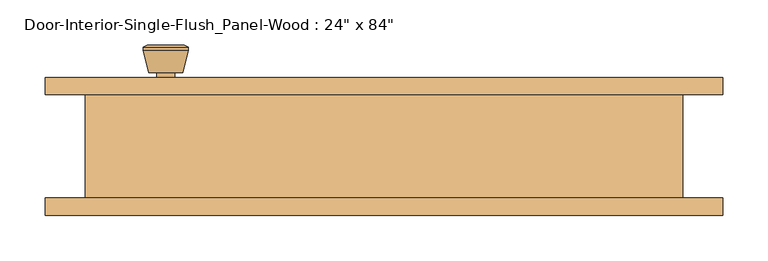
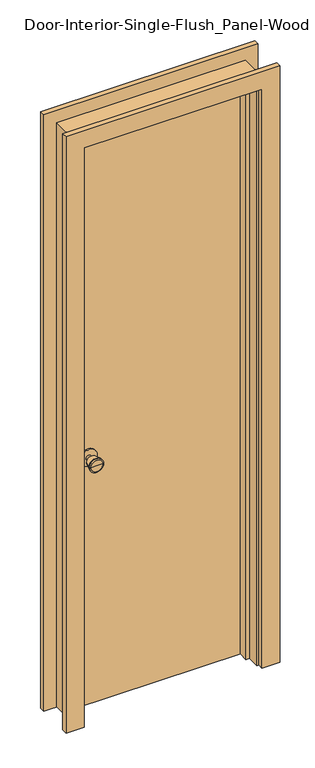
"""IFC4 building model written with IfcOpenShell, lengths in millimetres: door geometry."""

from ifc_helpers import new_model, si_unit, point, frame, frame_2d, origin, origin_with_axes, place, context, project, spatial, polyline, circle_curve, trimmed, segment, composite_curve, outline, extrude, faceted_brep, source, transform, mapped, element, save
from ifc_brep_helpers import plane_surface, cylinder_surface, revolved_surface, advanced_brep


def door_c25f678d(model_context):
    return source(origin(), model_context, "Body", "SolidModel", [
        advanced_brep(
        [(-241.3, 13.05, 914.4), (-231.3, 13.05, 914.4), (-251.3, 13.05, 914.4), (-220.8241324, -35.95, 914.4), (-241.3, -35.95, 914.4), (-261.7758676, -35.95, 914.4), (-216.3, -34.1221319, 914.4), (-266.3, -34.1221319, 914.4), (-216.3, -30.6584537, 914.4), (-266.3, -30.6584537, 914.4), (-222.663764, -5.95, 914.4), (-259.936236, -5.95, 914.4), (-231.3, -5.95, 914.4), (-251.3, -5.95, 914.4)],
        [
            (0, 1),
            (1, 2, circle_curve(frame((-241.3, 13.05, 914.4), z_axis=(0.0, 1.0, 0.0), x_axis=(-1.0, 0.0, 0.0)), 10.0)),
            (2, 0),
            (2, 1, circle_curve(frame((-241.3, 13.05, 914.4), z_axis=(0.0, 1.0, 0.0), x_axis=(-1.0, 0.0, 0.0)), 10.0)),
            (3, 4),
            (4, 5),
            (5, 3, circle_curve(frame((-241.3, -35.95, 914.4), z_axis=(0.0, -1.0, 0.0), x_axis=(-1.0, 0.0, 0.0)), 20.4758676)),
            (3, 5, circle_curve(frame((-241.3, -35.95, 914.4), z_axis=(0.0, -1.0, 0.0), x_axis=(-1.0, 0.0, 0.0)), 20.4758676)),
            (6, 3),
            (5, 7),
            (7, 6, circle_curve(frame((-241.3, -34.1221319, 914.4), z_axis=(0.0, -1.0, 0.0), x_axis=(-1.0, 0.0, 0.0)), 25.0)),
            (6, 7, circle_curve(frame((-241.3, -34.1221319, 914.4), z_axis=(0.0, -1.0, 0.0), x_axis=(-1.0, 0.0, 0.0)), 25.0)),
            (8, 6),
            (7, 9),
            (9, 8, circle_curve(frame((-241.3, -30.6584537, 914.4), z_axis=(0.0, -1.0, 0.0), x_axis=(-1.0, 0.0, 0.0)), 25.0)),
            (8, 9, circle_curve(frame((-241.3, -30.6584537, 914.4), z_axis=(0.0, -1.0, 0.0), x_axis=(-1.0, 0.0, 0.0)), 25.0)),
            (10, 8),
            (9, 11),
            (11, 10, circle_curve(frame((-241.3, -5.95, 914.4), z_axis=(0.0, -1.0, 0.0), x_axis=(-1.0, 0.0, 0.0)), 18.636236)),
            (10, 11, circle_curve(frame((-241.3, -5.95, 914.4), z_axis=(0.0, -1.0, 0.0), x_axis=(-1.0, 0.0, 0.0)), 18.636236)),
            (12, 10),
            (11, 13),
            (13, 12, circle_curve(frame((-241.3, -5.95, 914.4), z_axis=(0.0, -1.0, 0.0), x_axis=(-1.0, 0.0, 0.0)), 10.0)),
            (12, 13, circle_curve(frame((-241.3, -5.95, 914.4), z_axis=(0.0, -1.0, 0.0), x_axis=(-1.0, 0.0, 0.0)), 10.0)),
            (1, 12),
            (13, 2),
        ],
        [
            plane_surface(frame((-241.3, 13.05, 914.4), z_axis=(0.0, 1.0, 0.0), x_axis=(-1.0, 0.0, 0.0))),
            plane_surface(frame((-241.3, -35.95, 914.4), z_axis=(0.0, -1.0, 0.0), x_axis=(-1.0, 0.0, 0.0))),
            revolved_surface(polyline([(-261.7758676, -35.95, 914.4), (-266.3, -34.1221319, 914.4)]), (-241.3, 13.05, 914.4), (0.0, 1.0, 0.0)),
            cylinder_surface(frame((-241.3, 13.05, 914.4), z_axis=(0.0, 1.0, 0.0), x_axis=(-1.0, 0.0, 0.0)), 25.0),
            revolved_surface(polyline([(-266.3, -30.6584537, 914.4), (-259.936236, -5.95, 914.4)]), (-241.3, 13.05, 914.4), (0.0, 1.0, 0.0)),
            plane_surface(frame((-241.3, -5.95, 914.4), z_axis=(0.0, 1.0, 0.0), x_axis=(-1.0, 0.0, 0.0))),
            cylinder_surface(frame((-241.3, 13.05, 914.4), z_axis=(0.0, 1.0, 0.0), x_axis=(-1.0, 0.0, 0.0)), 10.0),
        ],
        [
            (0, [[1, 2, 3]]),
            (0, [[-3, 4, -1]]),
            (1, [[5, 6, 7]]),
            (1, [[-6, -5, 8]]),
            (2, [[9, -7, 10, 11]]),
            (2, [[-10, -8, -9, 12]]),
            (3, [[13, -11, 14, 15]]),
            (3, [[-14, -12, -13, 16]]),
            (4, [[17, -15, 18, 19]]),
            (4, [[-18, -16, -17, 20]]),
            (5, [[21, -19, 22, 23]]),
            (5, [[-22, -20, -21, 24]]),
            (6, [[25, -23, 26, -2]]),
            (6, [[-26, -24, -25, -4]]),
        ],
    ),
        extrude(outline(composite_curve([segment(trimmed(circle_curve(frame_2d((914.4, -241.3)), 30.0), [point((914.4, -271.3))], [point((914.4, -211.3))], False, "CARTESIAN"), True, "CONTINUOUS"), segment(trimmed(circle_curve(frame_2d((914.4, -241.3)), 30.0), [point((914.4, -211.3))], [point((914.4, -271.3))], False, "CARTESIAN"), True, "CONTINUOUS")], self_intersect=False)), frame((0.0, 13.05, 0.0), z_axis=(0.0, 1.0, 0.0), x_axis=(0.0, 0.0, 1.0)), (0.0, 0.0, 1.0), 6.0),
        advanced_brep(
        [(-241.3, 59.975, 914.4), (-251.3, 59.975, 914.4), (-231.3, 59.975, 914.4), (-220.8241324, 108.975, 914.4), (-261.7758676, 108.975, 914.4), (-241.3, 108.975, 914.4), (-216.3, 107.1471319, 914.4), (-266.3, 107.1471319, 914.4), (-216.3, 103.6834537, 914.4), (-266.3, 103.6834537, 914.4), (-222.663764, 78.975, 914.4), (-259.936236, 78.975, 914.4), (-231.3, 78.975, 914.4), (-251.3, 78.975, 914.4)],
        [
            (0, 1),
            (1, 2, circle_curve(frame((-241.3, 59.975, 914.4), z_axis=(0.0, -1.0, 0.0), x_axis=(-1.0, 0.0, 0.0)), 10.0)),
            (2, 0),
            (2, 1, circle_curve(frame((-241.3, 59.975, 914.4), z_axis=(0.0, -1.0, 0.0), x_axis=(-1.0, 0.0, 0.0)), 10.0)),
            (3, 4, circle_curve(frame((-241.3, 108.975, 914.4), z_axis=(0.0, 1.0, 0.0), x_axis=(-1.0, 0.0, 0.0)), 20.4758676)),
            (4, 5),
            (5, 3),
            (4, 3, circle_curve(frame((-241.3, 108.975, 914.4), z_axis=(0.0, 1.0, 0.0), x_axis=(-1.0, 0.0, 0.0)), 20.4758676)),
            (6, 7, circle_curve(frame((-241.3, 107.1471319, 914.4), z_axis=(0.0, 1.0, 0.0), x_axis=(-1.0, 0.0, 0.0)), 25.0)),
            (7, 4),
            (3, 6),
            (7, 6, circle_curve(frame((-241.3, 107.1471319, 914.4), z_axis=(0.0, 1.0, 0.0), x_axis=(-1.0, 0.0, 0.0)), 25.0)),
            (8, 9, circle_curve(frame((-241.3, 103.6834537, 914.4), z_axis=(0.0, 1.0, 0.0), x_axis=(-1.0, 0.0, 0.0)), 25.0)),
            (9, 7),
            (6, 8),
            (9, 8, circle_curve(frame((-241.3, 103.6834537, 914.4), z_axis=(0.0, 1.0, 0.0), x_axis=(-1.0, 0.0, 0.0)), 25.0)),
            (10, 11, circle_curve(frame((-241.3, 78.975, 914.4), z_axis=(0.0, 1.0, 0.0), x_axis=(-1.0, 0.0, 0.0)), 18.636236)),
            (11, 9),
            (8, 10),
            (11, 10, circle_curve(frame((-241.3, 78.975, 914.4), z_axis=(0.0, 1.0, 0.0), x_axis=(-1.0, 0.0, 0.0)), 18.636236)),
            (12, 13, circle_curve(frame((-241.3, 78.975, 914.4), z_axis=(0.0, 1.0, 0.0), x_axis=(-1.0, 0.0, 0.0)), 10.0)),
            (13, 11),
            (10, 12),
            (13, 12, circle_curve(frame((-241.3, 78.975, 914.4), z_axis=(0.0, 1.0, 0.0), x_axis=(-1.0, 0.0, 0.0)), 10.0)),
            (1, 13),
            (12, 2),
        ],
        [
            plane_surface(frame((-241.3, 59.975, 914.4), z_axis=(0.0, -1.0, 0.0), x_axis=(-1.0, 0.0, 0.0))),
            plane_surface(frame((-241.3, 108.975, 914.4), z_axis=(0.0, 1.0, 0.0), x_axis=(-1.0, 0.0, 0.0))),
            revolved_surface(polyline([(-261.7758676, 108.975, 914.4), (-266.3, 107.1471319, 914.4)]), (-241.3, 59.975, 914.4), (0.0, -1.0, 0.0)),
            cylinder_surface(frame((-241.3, 59.975, 914.4), z_axis=(0.0, -1.0, 0.0), x_axis=(-1.0, 0.0, 0.0)), 25.0),
            revolved_surface(polyline([(-266.3, 103.6834537, 914.4), (-259.936236, 78.975, 914.4)]), (-241.3, 59.975, 914.4), (0.0, -1.0, 0.0)),
            plane_surface(frame((-241.3, 78.975, 914.4), z_axis=(0.0, -1.0, 0.0), x_axis=(-1.0, 0.0, 0.0))),
            cylinder_surface(frame((-241.3, 59.975, 914.4), z_axis=(0.0, -1.0, 0.0), x_axis=(-1.0, 0.0, 0.0)), 10.0),
        ],
        [
            (0, [[1, 2, 3]]),
            (0, [[-3, 4, -1]]),
            (1, [[5, 6, 7]]),
            (1, [[8, -7, -6]]),
            (2, [[9, 10, -5, 11]]),
            (2, [[12, -11, -8, -10]]),
            (3, [[13, 14, -9, 15]]),
            (3, [[16, -15, -12, -14]]),
            (4, [[17, 18, -13, 19]]),
            (4, [[20, -19, -16, -18]]),
            (5, [[21, 22, -17, 23]]),
            (5, [[24, -23, -20, -22]]),
            (6, [[-2, 25, -21, 26]]),
            (6, [[-4, -26, -24, -25]]),
        ],
    ),
        extrude(outline(composite_curve([segment(trimmed(circle_curve(frame_2d((914.4, -241.3)), 30.0), [point((914.4, -271.3))], [point((914.4, -211.3))], False, "CARTESIAN"), True, "CONTINUOUS"), segment(trimmed(circle_curve(frame_2d((914.4, -241.3)), 30.0), [point((914.4, -211.3))], [point((914.4, -271.3))], False, "CARTESIAN"), True, "CONTINUOUS")], self_intersect=False)), frame((0.0, 53.975, 0.0), z_axis=(0.0, 1.0, 0.0), x_axis=(0.0, 0.0, 1.0)), (0.0, 0.0, 1.0), 6.0),
        faceted_brep([(330.2, 53.975, 0.0), (330.2, -60.325, 0.0), (304.8, -60.325, 0.0), (304.8, -15.875, 0.0), (292.1, -15.875, 0.0), (292.1, 19.05, 0.0), (304.8, 19.05, 0.0), (304.8, 53.975, 0.0), (330.2, 53.975, 2159.0), (330.2, -60.325, 2159.0), (-330.2, -60.325, 2159.0), (-330.2, -60.325, 0.0), (-304.8, -60.325, 0.0), (-304.8, -60.325, 2133.6), (304.8, -60.325, 2133.6), (304.8, -15.875, 2133.6), (-304.8, -15.875, 2133.6), (-304.8, -15.875, 0.0), (-292.1, -15.875, 0.0), (-292.1, -15.875, 2120.9), (292.1, -15.875, 2120.9), (292.1, 19.05, 2120.9), (-292.1, 19.05, 2120.9), (-292.1, 19.05, 0.0), (-304.8, 19.05, 0.0), (-304.8, 19.05, 2133.6), (304.8, 19.05, 2133.6), (304.8, 53.975, 2133.6), (-304.8, 53.975, 2133.6), (-304.8, 53.975, 0.0), (-330.2, 53.975, 0.0), (-330.2, 53.975, 2159.0)], [[[0, 1, 2, 3, 4, 5, 6, 7]], [[1, 0, 8, 9]], [[2, 1, 9, 10, 11, 12, 13, 14]], [[3, 2, 14, 15]], [[4, 3, 15, 16, 17, 18, 19, 20]], [[5, 4, 20, 21]], [[6, 5, 21, 22, 23, 24, 25, 26]], [[7, 6, 26, 27]], [[0, 7, 27, 28, 29, 30, 31, 8]], [[9, 8, 31, 10]], [[15, 14, 13, 16]], [[21, 20, 19, 22]], [[27, 26, 25, 28]], [[30, 29, 24, 23, 18, 17, 12, 11]], [[10, 31, 30, 11]], [[16, 13, 12, 17]], [[22, 19, 18, 23]], [[28, 25, 24, 29]]]),
        extrude(outline(polyline([(304.8, 19.05), (-304.8, 19.05), (-304.8, 53.975), (304.8, 53.975), (304.8, 19.05)])), origin_with_axes(), (0.0, 0.0, 1.0), 2133.6),
        extrude(outline(polyline([(0.0, 311.15), (0.0, 374.65), (2203.45, 374.65), (2203.45, -374.65), (0.0, -374.65), (0.0, -311.15), (2139.95, -311.15), (2139.95, 311.15), (0.0, 311.15)])), frame((0.0, 53.975, 0.0), z_axis=(0.0, 1.0, 0.0), x_axis=(0.0, 0.0, 1.0)), (0.0, 0.0, 1.0), 19.05),
        extrude(outline(polyline([(0.0, 311.15), (0.0, 374.65), (2203.45, 374.65), (2203.45, -374.65), (0.0, -374.65), (0.0, -311.15), (2139.95, -311.15), (2139.95, 311.15), (0.0, 311.15)])), frame((0.0, -79.375, 0.0), z_axis=(0.0, 1.0, 0.0), x_axis=(0.0, 0.0, 1.0)), (0.0, 0.0, 1.0), 19.05),
    ])


if __name__ == "__main__":
    model = new_model("IFC4")
    model_context = context("Model", 3, world=origin())
    ifc_project = project(units=[si_unit("LENGTHUNIT", "METRE", prefix="MILLI")], contexts=[model_context])
    site = spatial("IfcSite", under=ifc_project)
    building = spatial("IfcBuilding", under=site)
    placement = place(None, origin())
    door_shape = door_c25f678d(model_context)
    element("IfcDoor", 1, ObjectType="Door-Interior-Single-Flush_Panel-Wood : 24\" x 84\"", at=placement, inside=building, context=model_context, shape_type="MappedRepresentation", body=[
        mapped(door_shape, transform((0.0, 0.0, 0.0), x_axis=(1.0, 0.0, 0.0), y_axis=(0.0, 1.0, 0.0), z_axis=(0.0, 0.0, 1.0))),
    ])
    save(model, "model.ifc")

# Revit data of these elements
# Type "Door-Interior-Single-Flush_Panel-Wood : 24\" x 84\""
#   Type Mark = "10"
#   Assembly Code = "C1020300"
#   Analytic Construction = "Wooden"
#   Thickness = 0' - 1 3/8"
#   Thermal Resistance (R) = 2.5876 (h·ft²·°F)/BTU
#   Swing Angle [instance default] = 90.00°
#   Rough Width = 2' - 2"
#   Rough Height = 7' - 1"
#   Height = 7' - 0"
#   Width = 2' - 0"
#   Heat Transfer Coefficient (U) = 0.3865 BTU/(h·ft²·°F)
#   Trim Material = Cherry
#   Panel Material = Cherry
#   Frame Material = Cherry
#   Door Handle Material = Aluminum
#   Visual Light Transmittance = 0
#   Solar Heat Gain Coefficient = 0
#   Wall Closure = (empty or 0)
#   Function = (empty or 0)
# Element 1 (IfcDoor, "Door-Interior-Single-Flush_Panel-Wood : 24\" x 84\"")
#   Materials on its faces: "Cherry", "Aluminum"
# Materials
#   "Cherry": class "Wood", colour RGB 226 177 128, transparency 0, Description = "Prunus Serotina", Cost = 0
#   "Aluminum": class "Metal", colour RGB 247 247 247, transparency 0, Description = "Aluminum 6061", Cost = 0
